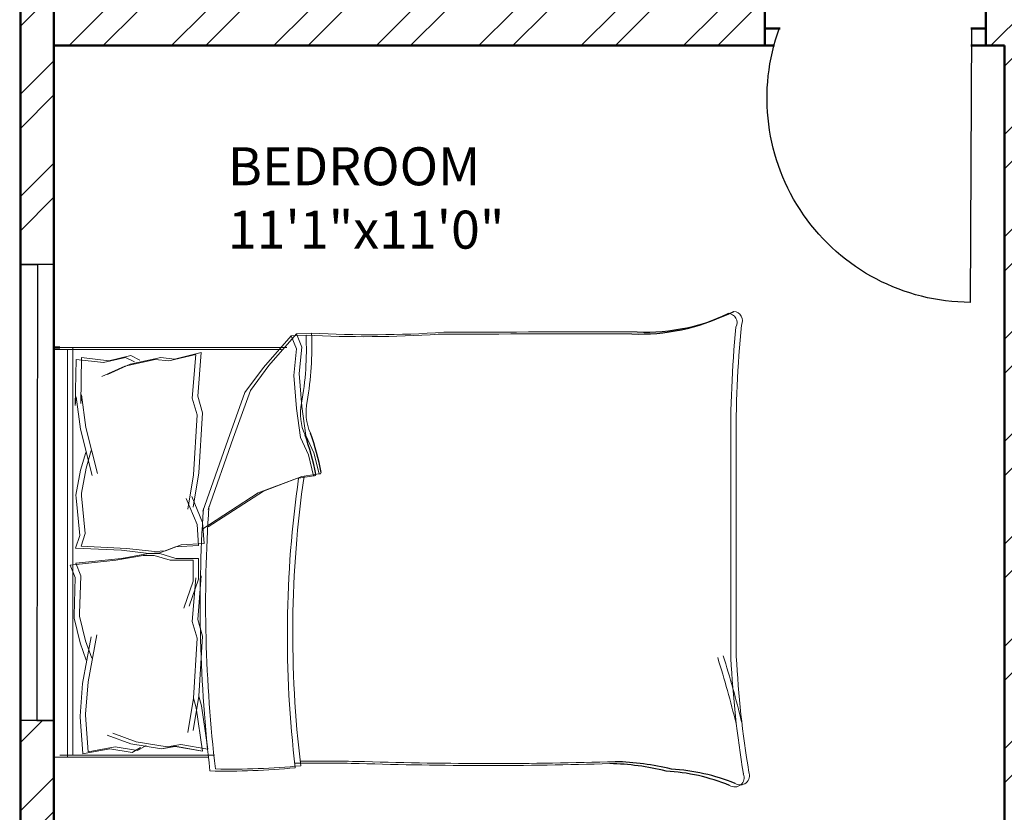
# Model space of a CAD drawing. Units: inches. Extents: x 1901 to 2863, y 888 to 2433.
# Tile 3 of 91: x 2025 to 2154, y 1338 to 1442. Entities that reach past the tile are written whole.
import ezdxf

# ---------------------------------------------------------------- set-up
doc = ezdxf.new("R2010")
doc.units = ezdxf.units.IN
for name, color, linetype, lineweight in [('A-AREA-IDEN', 7, 'Continuous', 18), ('A-DOOR', 4, 'Continuous', 25), ('A-FURN', 8, 'Continuous', 18), ('A-GLAZ', 3, 'Continuous', 25), ('A-WALL', 7, 'Continuous', 50), ('A-WALL-PATT', 8, 'Continuous', 13)]:
    doc.layers.add(name, color=color, linetype=linetype, lineweight=lineweight)
doc.styles.get("Standard").update_dxf_attribs({"font": 'arial.ttf'})

# ---------------------------------------------------------------- blocks, each defined once
blk = doc.blocks.new('WIN-60')
for p, q in [((0, 4.5), (0, 0)), ((60, 2.25), (60, 4.5)), ((60, 4.5), (60, 0)), ((0, 0), (0, 2.25)), ((0, 2.25), (60, 2.25))]:
    blk.add_line(p, q)
blk = doc.blocks.new('DOOR-27')
blk.add_line((26.81, -0.02), (26.81, 35.98))
blk.add_arc((26.81, 9.12), 26.86, 90, 199.8893)

msp = doc.modelspace()

# ---------------------------------------------------------------- hatches: boundary and pattern name
at = {"layer": 'A-WALL-PATT'}
h = msp.add_hatch(dxfattribs=at)
h.set_pattern_fill('ANSI32', color=256)
h.paths.add_polyline_path([(2192.5, 2274.13), (2141.26, 2274.13), (2141.26, 2269.63), (2192.5, 2269.63)])
h.paths.add_polyline_path([(2259.93, 2274.13), (2216.5, 2274.13), (2216.5, 2269.63), (2255.43, 2269.63), (2255.43, 2214.63), (2250.81, 2214.63), (2250.81, 2210.13), (2259.93, 2210.13), (2259.93, 2215.13), (2271.76, 2215.13), (2271.76, 2217.38), (2271.76, 2219.63), (2259.93, 2219.63)])
h.paths.add_polyline_path([(2171.43, 2269.63), (2166.93, 2269.63), (2166.93, 2219.63), (2121.24, 2219.63), (2121.24, 2215.13), (2166.93, 2215.13), (2166.93, 2083.13), (2161.81, 2083.13), (2161.81, 2078.63), (2171.43, 2078.63), (2177, 2078.63), (2177, 2080.88), (2177, 2083.13), (2171.43, 2083.13), (2171.43, 2210.13), (2230.91, 2210.13), (2230.91, 2212.38), (2230.91, 2214.63), (2171.43, 2214.63)])
h.paths.add_polyline_path([(2117.26, 2274.13), (2089.43, 2274.13), (2089.43, 2219.63), (2081.14, 2219.63), (2081.14, 2215.13), (2089.43, 2215.13), (2098, 2215.13), (2098, 2217.38), (2098, 2219.63), (2093.93, 2219.63), (2093.93, 2269.63), (2117.26, 2269.63), (2117.26, 2271.88)])
h.paths.add_polyline_path([(2343.43, 2219.63), (2329.29, 2219.63), (2329.29, 2215.13), (2338.93, 2215.13), (2338.93, 2184.74), (2343.43, 2184.74)])
h.paths.add_polyline_path([(2338.93, 2083.13), (2329.29, 2083.13), (2208.97, 2083.13), (2208.97, 2078.63), (2338.93, 2078.63)])
h.paths.add_polyline_path([(2343.43, 2136.74), (2338.93, 2136.74), (2338.93, 1872.63), (2343.43, 1872.63)])
h.paths.add_polyline_path([(2343.43, 1863.63), (2397.68, 1863.63), (2397.68, 1821.63), (2384.14, 1821.63), (2384.14, 1812.63), (2418.33, 1812.63), (2418.33, 1817.13), (2418.33, 1821.63), (2406.68, 1821.63), (2406.68, 1863.63), (2459.5, 1863.63), (2459.5, 1821.63), (2447.14, 1821.63), (2447.14, 1812.63), (2459.5, 1812.63), (2468.5, 1812.63), (2468.5, 1872.63), (2394.43, 1872.63), (2334.43, 1872.63), (2334.43, 1812.63), (2343.43, 1812.63), (2353.25, 1812.63), (2353.25, 1821.63), (2343.43, 1821.63)])
h.paths.add_polyline_path([(2510.01, 1872.63), (2468.5, 1872.63), (2468.5, 1868.13), (2510.01, 1868.13)])
h.paths.add_polyline_path([(2514.01, 1817.13), (2468.5, 1817.13), (2468.5, 1812.63), (2482.11, 1812.63), (2482.11, 1800.61), (2486.61, 1800.61), (2486.61, 1812.63), (2514.01, 1812.63)])
h.paths.add_polyline_path([(2299.25, 1814.88), (2299.25, 1817.13), (2295.93, 1817.13), (2295.93, 1854.17), (2293.68, 1854.17), (2291.43, 1854.17), (2291.43, 1817.13), (2266.11, 1817.13), (2266.11, 1812.63), (2299.25, 1812.63)])
h.paths.add_polyline_path([(2218.11, 1817.13), (2206.46, 1817.13), (2171.43, 1817.13), (2171.43, 1949.13), (2190.1, 1949.13), (2190.1, 1953.63), (2163.47, 1953.63), (2163.47, 1949.13), (2166.93, 1949.13), (2166.93, 1817.13), (2114.3, 1817.13), (2114.3, 1812.63), (2218.11, 1812.63)])
h.paths.add_polyline_path([(2029.43, 1970.92), (2024.93, 1970.92), (2024.93, 1912.72), (2029.43, 1912.72)])
h.paths.add_polyline_path([(2132.3, 1953.63), (2113.93, 1953.63), (2113.93, 1975.89), (2111.68, 1975.89), (2109.43, 1975.89), (2109.43, 1953.63), (2029.43, 1953.63), (2029.43, 1949.13), (2132.3, 1949.13)])
h.paths.add_polyline_path([(2029.43, 1853.61), (2029.31, 1853.61), (2029.31, 1853.61), (2029.43, 1853.61), (2029.43, 1864.72), (2024.93, 1864.72), (2024.93, 1812.63), (2066.3, 1812.63), (2066.3, 1814.88), (2066.3, 1817.13), (2029.43, 1817.13)])
h.paths.add_polyline_path([(2122.93, 2010.09), (2120.68, 2010.09), (2118.43, 2010.09), (2118.43, 2006.13), (2029.43, 2006.13), (2029.43, 2001.63), (2109.43, 2001.63), (2109.43, 1998.04), (2113.93, 1998.04), (2113.93, 2001.63), (2122.93, 2001.63)])
h.paths.add_polyline_path([(2029.43, 2031.38), (2024.93, 2031.38), (2024.93, 1994.92), (2027.18, 1994.92), (2029.43, 1994.92)])
h.paths.add_polyline_path([(2029.43, 2136.74), (2024.93, 2136.74), (2024.93, 2067.38), (2027.18, 2067.38), (2029.43, 2067.38)])
h.paths.add_polyline_path([(2125.62, 2083.13), (2029.43, 2083.13), (2029.43, 2078.63), (2118.43, 2078.63), (2118.43, 2030.71), (2122.93, 2030.71), (2122.93, 2078.63), (2125.62, 2078.63)])
h.paths.add_polyline_path([(2029.43, 2215.13), (2040.47, 2215.13), (2040.47, 2217.38), (2040.47, 2219.63), (2024.93, 2219.63), (2024.93, 2184.74), (2029.43, 2184.74), (2029.43, 2187.78)])
h.paths.add_polyline_path([(2686.43, 2274.13), (2659.28, 2274.13), (2659.28, 2269.63), (2681.93, 2269.63), (2681.93, 2219.63), (2676.82, 2219.63), (2676.82, 2215.13), (2681.93, 2215.13), (2697.01, 2215.13), (2697.01, 2217.38), (2697.01, 2219.63), (2686.43, 2219.63)])
h.paths.add_polyline_path([(2609.93, 2269.63), (2635.28, 2269.63), (2635.28, 2274.13), (2571.43, 2274.13), (2571.43, 2269.63), (2605.43, 2269.63), (2605.43, 2214.63), (2549.1, 2214.63), (2549.1, 2210.13), (2605.43, 2210.13), (2605.43, 2083.13), (2601.01, 2083.13), (2601.01, 2080.88), (2601.01, 2078.63), (2609.93, 2078.63), (2616.16, 2078.63), (2616.16, 2080.88), (2616.16, 2083.13), (2609.93, 2083.13), (2609.93, 2215.13), (2651.46, 2215.13), (2651.46, 2217.38), (2651.46, 2219.63), (2609.93, 2219.63)])
h.paths.add_polyline_path([(2521.43, 2269.63), (2547.43, 2269.63), (2547.43, 2271.88), (2547.43, 2274.13), (2516.93, 2274.13), (2516.93, 2219.63), (2506.41, 2219.63), (2506.41, 2215.13), (2516.93, 2215.13), (2516.93, 2210.13), (2525.4, 2210.13), (2525.4, 2212.38), (2525.4, 2214.63), (2521.43, 2214.63)])
h.paths.add_polyline_path([(2456.01, 2219.63), (2439.43, 2219.63), (2439.43, 2187.89), (2443.93, 2187.89), (2443.93, 2215.13), (2456.01, 2215.13)])
h.paths.add_polyline_path([(2752.93, 2219.63), (2739.48, 2219.63), (2739.48, 2215.13), (2748.43, 2215.13), (2748.43, 2187.89), (2752.93, 2187.89)])
h.paths.add_polyline_path([(2752.93, 2139.89), (2748.43, 2139.89), (2748.43, 2083.13), (2648.42, 2083.13), (2648.42, 2078.63), (2654.93, 2078.63), (2654.93, 2039.44), (2659.43, 2039.44), (2659.43, 2078.63), (2748.43, 2078.63), (2748.43, 2063.43), (2752.93, 2063.43)])
h.paths.add_polyline_path([(2752.93, 2010.63), (2659.43, 2010.63), (2659.43, 2015.65), (2654.93, 2015.65), (2654.93, 2010.63), (2605.43, 2010.63), (2605.43, 1920.97), (2609.93, 1920.97), (2609.93, 2006.13), (2748.43, 2006.13), (2748.43, 1982.47), (2752.93, 1982.47)])
h.paths.add_polyline_path([(2752.93, 2027.43), (2748.43, 2027.43), (2748.43, 2010.63), (2752.93, 2010.63)])
h.paths.add_polyline_path([(2748.43, 1886.13), (2609.93, 1886.13), (2609.93, 1889.72), (2605.43, 1889.72), (2605.43, 1861.26), (2609.93, 1861.26), (2609.93, 1881.63), (2748.43, 1881.63)])
h.paths.add_polyline_path([(2456.86, 2228.83), (2498.4, 2228.83), (2498.4, 2247.49), (2456.86, 2247.49)], flags=9)
h.paths.add_polyline_path([(2038.6, 2237.42), (2080.17, 2237.42), (2080.17, 2256.08), (2038.6, 2256.08)], flags=9)
h.paths.add_polyline_path([(2292.01, 1062.39), (2539.93, 1062.39), (2539.93, 1099.49), (2292.01, 1099.49)], flags=9)
h.paths.add_polyline_path([(2424.91, 1832.25), (2448.51, 1832.25), (2448.51, 1846.68), (2424.91, 1846.68)], flags=25)
h.paths.add_polyline_path([(2359.08, 1832.25), (2382.68, 1832.25), (2382.68, 1846.68), (2359.08, 1846.68)], flags=25)
h.paths.add_polyline_path([(2352.9, 1684.8), (2367.54, 1684.8), (2367.54, 1697.17), (2352.9, 1697.17)], flags=9)
h.paths.add_polyline_path([(2079.29, 1755.83), (2169.02, 1755.83), (2169.02, 1774.37), (2079.29, 1774.37)], flags=9)
h.paths.add_polyline_path([(2404.09, 1373.86), (2404.09, 1463.59), (2385.54, 1463.59), (2385.54, 1373.86)], flags=9)
h.paths.add_polyline_path([(2268.09, 2236.37), (2309.64, 2236.37), (2309.64, 2255.03), (2268.09, 2255.03)], flags=9)
h.paths.add_polyline_path([(2575.96, 1700.95), (2665.7, 1700.95), (2665.7, 1719.5), (2575.96, 1719.5)], flags=9)
h.paths.add_polyline_path([(2302.96, 1878.47), (2329.52, 1878.47), (2329.52, 1888.78), (2302.96, 1888.78)], flags=9)
h.paths.add_polyline_path([(2097.42, 2240.58), (2126.57, 2240.58), (2126.57, 2259.23), (2097.42, 2259.23)], flags=9)
h.paths.add_polyline_path([(2208.72, 2246.12), (2237.88, 2246.12), (2237.88, 2264.78), (2208.72, 2264.78)], flags=9)
h.paths.add_polyline_path([(2038.15, 1925.96), (2076.99, 1925.96), (2076.99, 1944.62), (2038.15, 1944.62)], flags=9)
h.paths.add_polyline_path([(2239.14, 1926.67), (2288.46, 1926.67), (2288.46, 1945.33), (2239.14, 1945.33)], flags=9)
h.paths.add_polyline_path([(2175.43, 2007.33), (2212.36, 2007.33), (2212.36, 2025.99), (2175.43, 2025.99)], flags=9)
h.paths.add_polyline_path([(2225.03, 2091.79), (2263.87, 2091.79), (2263.87, 2110.45), (2225.03, 2110.45)], flags=9)
h.paths.add_polyline_path([(2035.4, 2098.48), (2074.24, 2098.48), (2074.24, 2117.14), (2035.4, 2117.14)], flags=9)
h.paths.add_polyline_path([(2050.1, 2029.21), (2083.26, 2029.21), (2083.26, 2047.87), (2050.1, 2047.87)], flags=9)
h.paths.add_polyline_path([(2069.68, 1956.72), (2098.83, 1956.72), (2098.83, 1975.38), (2069.68, 1975.38)], flags=25)
h.paths.add_polyline_path([(2328.62, 1753.34), (2361.66, 1753.34), (2361.66, 1771.99), (2328.62, 1771.99)], flags=9)
h.paths.add_polyline_path([(2395.16, 2060.89), (2395.16, 2140.65), (2378.68, 2140.65), (2378.68, 2060.89)], flags=9)
h.paths.add_polyline_path([(2463.73, 2059.02), (2492.89, 2059.02), (2492.89, 2077.68), (2463.73, 2077.68)], flags=9)
h.paths.add_polyline_path([(2458.03, 2181.54), (2496.87, 2181.54), (2496.87, 2200.19), (2458.03, 2200.19)], flags=9)
h.paths.add_polyline_path([(2527.58, 2243.07), (2556.73, 2243.07), (2556.73, 2261.73), (2527.58, 2261.73)], flags=9)
h.paths.add_polyline_path([(2694.46, 2232.77), (2736.03, 2232.77), (2736.03, 2251.42), (2694.46, 2251.42)], flags=9)
h.paths.add_polyline_path([(2637.82, 2249.22), (2666.98, 2249.22), (2666.98, 2267.88), (2637.82, 2267.88)], flags=9)
h.paths.add_polyline_path([(2623.69, 2183.54), (2662.53, 2183.54), (2662.53, 2202.2), (2623.69, 2202.2)], flags=9)
h.paths.add_polyline_path([(2691.97, 2021.5), (2725.12, 2021.5), (2725.12, 2040.16), (2691.97, 2040.16)], flags=9)
h.paths.add_polyline_path([(2621.04, 1975.91), (2662.34, 1975.91), (2662.34, 1994.57), (2621.04, 1994.57)], flags=25)
h.paths.add_polyline_path([(2479.03, 1927.62), (2519.84, 1927.62), (2519.84, 1946.28), (2479.03, 1946.28)], flags=9)
h.paths.add_polyline_path([(2670.94, 1849.08), (2716.01, 1849.08), (2716.01, 1867.73), (2670.94, 1867.73)], flags=9)
h.paths.add_polyline_path([(2523.61, 1782.96), (2550.17, 1782.96), (2550.17, 1793.26), (2523.61, 1793.26)], flags=9)
h.paths.add_polyline_path([(2450.84, 1207.33), (2492.39, 1207.33), (2492.39, 1225.99), (2450.84, 1225.99)], flags=9)
h.paths.add_polyline_path([(2527.75, 1203.84), (2556.91, 1203.84), (2556.91, 1222.5), (2527.75, 1222.5)], flags=9)
h.paths.add_polyline_path([(2639.11, 1207.2), (2668.27, 1207.2), (2668.27, 1225.86), (2639.11, 1225.86)], flags=9)
h.paths.add_polyline_path([(2692.59, 1218.97), (2734.17, 1218.97), (2734.17, 1237.62), (2692.59, 1237.62)], flags=9)
h.paths.add_polyline_path([(2669.27, 1366.33), (2708.11, 1366.33), (2708.11, 1384.99), (2669.27, 1384.99)], flags=9)
h.paths.add_polyline_path([(2463.31, 1358.03), (2502.15, 1358.03), (2502.15, 1376.69), (2463.31, 1376.69)], flags=9)
h.paths.add_polyline_path([(2494.72, 1449.96), (2531.65, 1449.96), (2531.65, 1468.62), (2494.72, 1468.62)], flags=9)
h.paths.add_polyline_path([(2675.57, 1422.16), (2708.72, 1422.16), (2708.72, 1440.81), (2675.57, 1440.81)], flags=9)
h.paths.add_polyline_path([(2685.63, 1493.89), (2714.79, 1493.89), (2714.79, 1512.55), (2685.63, 1512.55)], flags=9)
h.paths.add_polyline_path([(2686.8, 1529.91), (2725.65, 1529.91), (2725.65, 1548.57), (2686.8, 1548.57)], flags=9)
h.paths.add_polyline_path([(2503.65, 1537.99), (2552.97, 1537.99), (2552.97, 1556.65), (2503.65, 1556.65)], flags=9)
h.paths.add_polyline_path([(2291.71, 1643.5), (2318.28, 1643.5), (2318.28, 1653.81), (2291.71, 1653.81)], flags=9)
h.paths.add_polyline_path([(2450.63, 1610.52), (2477.19, 1610.52), (2477.19, 1620.82), (2450.63, 1620.82)], flags=9)
h.paths.add_polyline_path([(2359.99, 1551.81), (2422.25, 1551.81), (2422.25, 1562.12), (2359.99, 1562.12)], flags=9)
h.paths.add_polyline_path([(2280.11, 1249.01), (2321.65, 1249.01), (2321.65, 1267.66), (2280.11, 1267.66)], flags=9)
h.paths.add_polyline_path([(2164.06, 1274.23), (2193.22, 1274.23), (2193.22, 1292.89), (2164.06, 1292.89)], flags=9)
h.paths.add_polyline_path([(2118.21, 1277.69), (2151.25, 1277.69), (2151.25, 1296.35), (2118.21, 1296.35)], flags=9)
h.paths.add_polyline_path([(2031.95, 1268.53), (2073.52, 1268.53), (2073.52, 1287.19), (2031.95, 1287.19)], flags=9)
h.paths.add_polyline_path([(2050.2, 1409.08), (2089.04, 1409.08), (2089.04, 1427.74), (2050.2, 1427.74)], flags=9)
h.paths.add_polyline_path([(2243.74, 1421.03), (2282.58, 1421.03), (2282.58, 1439.69), (2243.74, 1439.69)], flags=9)
h.paths.add_polyline_path([(2190.75, 1509.77), (2231.56, 1509.77), (2231.56, 1528.43), (2190.75, 1528.43)], flags=9)
h.paths.add_polyline_path([(2058.39, 1475.42), (2091.55, 1475.42), (2091.55, 1494.07), (2058.39, 1494.07)], flags=9)
h.paths.add_polyline_path([(2062.45, 1553.09), (2091.6, 1553.09), (2091.6, 1571.75), (2062.45, 1571.75)], flags=9)
h.paths.add_polyline_path([(2219.52, 1590.37), (2266.15, 1590.37), (2266.15, 1609.02), (2219.52, 1609.02)], flags=9)
h.paths.add_polyline_path([(2041.07, 1584.19), (2079.91, 1584.19), (2079.91, 1602.85), (2041.07, 1602.85)], flags=9)
h = msp.add_hatch(dxfattribs=at)
h.set_pattern_fill('ANSI32', color=256)
h.paths.add_polyline_path([(2443.93, 2139.89), (2439.43, 2139.89), (2439.43, 2069.35), (2441.68, 2069.35), (2443.93, 2069.35), (2443.93, 2078.63), (2521.93, 2078.63), (2521.93, 2075.07), (2524.18, 2075.07), (2526.43, 2075.07), (2526.43, 2078.63), (2571.75, 2078.63), (2571.75, 2080.88), (2571.75, 2083.13), (2443.93, 2083.13)])
h.paths.add_polyline_path([(2526.43, 2054.63), (2524.18, 2054.63), (2521.93, 2054.63), (2521.93, 2030.63), (2443.93, 2030.63), (2443.93, 2045.35), (2439.43, 2045.35), (2439.43, 1983.87), (2443.93, 1983.87), (2443.93, 2026.13), (2521.93, 2026.13), (2526.43, 2026.13)])
h.paths.add_polyline_path([(2443.93, 1923.87), (2439.43, 1923.87), (2439.43, 1872.63), (2443.93, 1872.63)])
h.paths.add_polyline_path([(2636.23, 1766.13), (2609.93, 1766.13), (2609.93, 1779.79), (2605.43, 1779.79), (2605.43, 1766.13), (2486.61, 1766.13), (2486.61, 1770.67), (2482.11, 1770.67), (2482.11, 1766.13), (2482.11, 1761.63), (2636.23, 1761.63), (2636.23, 1763.88)])
h.paths.add_polyline_path([(2519.54, 1663.38), (2519.54, 1665.63), (2494.93, 1665.63), (2481.83, 1665.63), (2481.83, 1663.38), (2481.83, 1661.13), (2490.43, 1661.13), (2490.43, 1640.16), (2494.93, 1640.16), (2494.93, 1661.13), (2519.54, 1661.13)])
h.paths.add_polyline_path([(2443.93, 1712.13), (2443.93, 1716.63), (2414.46, 1716.63), (2414.46, 1712.13), (2439.43, 1712.13), (2439.43, 1545.51), (2443.93, 1545.51), (2443.93, 1661.13), (2448.47, 1661.13), (2448.47, 1665.63), (2443.93, 1665.63)])
h.paths.add_polyline_path([(2343.43, 1712.13), (2365.52, 1712.13), (2365.52, 1714.38), (2365.52, 1716.63), (2333.87, 1716.63), (2333.87, 1714.38), (2333.87, 1712.13), (2338.93, 1712.13), (2338.93, 1575.63), (2338.93, 1545.51), (2343.43, 1545.51), (2343.43, 1547.51), (2343.43, 1580.13)])
h.paths.add_polyline_path([(2752.93, 1665.63), (2579.54, 1665.63), (2579.54, 1661.13), (2615.93, 1661.13), (2615.93, 1529.13), (2598.93, 1529.13), (2598.93, 1524.63), (2623.13, 1524.63), (2623.13, 1526.88), (2623.13, 1529.13), (2620.43, 1529.13), (2620.43, 1661.13), (2748.43, 1661.13), (2748.43, 1633.5), (2752.93, 1633.5)])
h.paths.add_polyline_path([(2752.93, 1419.93), (2748.43, 1419.93), (2748.43, 1400.13), (2659.43, 1400.13), (2659.43, 1444.33), (2657.18, 1444.33), (2654.93, 1444.33), (2654.93, 1400.13), (2643.65, 1400.13), (2643.65, 1395.63), (2748.43, 1395.63), (2748.43, 1364.04), (2752.93, 1364.04)])
h.paths.add_polyline_path([(2752.93, 1492.88), (2748.43, 1492.88), (2748.43, 1476.63), (2667.43, 1476.63), (2667.43, 1479.71), (2665.18, 1479.71), (2662.93, 1479.71), (2662.93, 1476.63), (2654.93, 1476.63), (2654.93, 1469.54), (2659.43, 1469.54), (2659.43, 1472.13), (2748.43, 1472.13), (2748.43, 1455.93), (2752.93, 1455.93)])
h.paths.add_polyline_path([(2752.93, 1304.04), (2748.43, 1304.04), (2748.43, 1263.63), (2738.66, 1263.63), (2738.66, 1259.13), (2752.93, 1259.13)])
h.paths.add_polyline_path([(2685.93, 1259.13), (2695.49, 1259.13), (2695.49, 1261.38), (2695.49, 1263.63), (2677.84, 1263.63), (2677.84, 1261.38), (2677.84, 1259.13), (2681.43, 1259.13), (2681.43, 1203.63), (2653.28, 1203.63), (2653.28, 1199.13), (2685.93, 1199.13), (2685.93, 1203.63)])
h.paths.add_polyline_path([(2609.43, 1395.63), (2611.85, 1395.63), (2611.85, 1400.13), (2598.89, 1400.13), (2598.89, 1397.88), (2598.89, 1395.63), (2604.93, 1395.63), (2604.93, 1268.13), (2554.73, 1268.13), (2554.73, 1265.88), (2554.73, 1263.63), (2604.93, 1263.63), (2604.93, 1203.63), (2571.31, 1203.63), (2571.31, 1199.13), (2604.93, 1199.13), (2629.28, 1199.13), (2629.28, 1201.38), (2629.28, 1203.63), (2609.43, 1203.63), (2609.43, 1258.63), (2609.43, 1259.13), (2654.8, 1259.13), (2654.8, 1263.63), (2609.43, 1263.63)])
h.paths.add_polyline_path([(2443.93, 1304.04), (2439.43, 1304.04), (2439.43, 1259.13), (2443.93, 1259.13), (2456.16, 1259.13), (2456.16, 1261.38), (2456.16, 1263.63), (2443.93, 1263.63)])
h.paths.add_polyline_path([(2525.43, 1263.63), (2531.78, 1263.63), (2531.78, 1268.13), (2520.93, 1268.13), (2520.93, 1263.63), (2511.41, 1263.63), (2511.41, 1259.13), (2520.93, 1259.13), (2520.93, 1199.13), (2547.31, 1199.13), (2547.31, 1201.38), (2547.31, 1203.63), (2525.43, 1203.63)])
h.paths.add_polyline_path([(2443.93, 1434.84), (2439.43, 1434.84), (2439.43, 1364.04), (2441.68, 1364.04), (2443.93, 1364.04)])
h.paths.add_polyline_path([(2567.13, 1400.13), (2443.93, 1400.13), (2443.93, 1395.63), (2567.13, 1395.63)])
h.paths.add_polyline_path([(2443.93, 1545.51), (2439.43, 1545.51), (2439.43, 1494.84), (2443.93, 1494.84)])
h.paths.add_polyline_path([(2494.93, 1553.35), (2492.68, 1553.35), (2490.43, 1553.35), (2490.43, 1524.63), (2494.93, 1524.63), (2525.94, 1524.63), (2525.94, 1526.88), (2525.94, 1529.13), (2494.93, 1529.13)])
h.paths.add_polyline_path([(2752.93, 1573.5), (2748.43, 1573.5), (2748.43, 1529.13), (2657.76, 1529.13), (2657.76, 1524.63), (2662.93, 1524.63), (2662.93, 1498.63), (2667.43, 1498.63), (2667.43, 1524.63), (2748.43, 1524.63), (2748.43, 1516.88), (2752.93, 1516.88)])
h.paths.add_polyline_path([(2038.6, 2237.42), (2080.17, 2237.42), (2080.17, 2256.08), (2038.6, 2256.08)], flags=9)
h.paths.add_polyline_path([(2292.01, 1062.39), (2539.93, 1062.39), (2539.93, 1099.49), (2292.01, 1099.49)], flags=9)
h.paths.add_polyline_path([(2424.91, 1832.25), (2448.51, 1832.25), (2448.51, 1846.68), (2424.91, 1846.68)], flags=9)
h.paths.add_polyline_path([(2359.08, 1832.25), (2382.68, 1832.25), (2382.68, 1846.68), (2359.08, 1846.68)], flags=9)
h.paths.add_polyline_path([(2352.9, 1684.8), (2367.54, 1684.8), (2367.54, 1697.17), (2352.9, 1697.17)], flags=9)
h.paths.add_polyline_path([(2079.29, 1755.83), (2169.02, 1755.83), (2169.02, 1774.37), (2079.29, 1774.37)], flags=9)
h.paths.add_polyline_path([(2404.09, 1373.86), (2404.09, 1463.59), (2385.54, 1463.59), (2385.54, 1373.86)], flags=9)
h.paths.add_polyline_path([(2268.09, 2236.37), (2309.64, 2236.37), (2309.64, 2255.03), (2268.09, 2255.03)], flags=9)
h.paths.add_polyline_path([(2575.96, 1700.95), (2665.7, 1700.95), (2665.7, 1719.5), (2575.96, 1719.5)], flags=9)
h.paths.add_polyline_path([(2302.96, 1878.47), (2329.52, 1878.47), (2329.52, 1888.78), (2302.96, 1888.78)], flags=9)
h.paths.add_polyline_path([(2097.42, 2240.58), (2126.57, 2240.58), (2126.57, 2259.23), (2097.42, 2259.23)], flags=9)
h.paths.add_polyline_path([(2208.72, 2246.12), (2237.88, 2246.12), (2237.88, 2264.78), (2208.72, 2264.78)], flags=9)
h.paths.add_polyline_path([(2038.15, 1925.96), (2076.99, 1925.96), (2076.99, 1944.62), (2038.15, 1944.62)], flags=9)
h.paths.add_polyline_path([(2239.14, 1926.67), (2288.46, 1926.67), (2288.46, 1945.33), (2239.14, 1945.33)], flags=9)
h.paths.add_polyline_path([(2175.43, 2007.33), (2212.36, 2007.33), (2212.36, 2025.99), (2175.43, 2025.99)], flags=9)
h.paths.add_polyline_path([(2225.03, 2091.79), (2263.87, 2091.79), (2263.87, 2110.45), (2225.03, 2110.45)], flags=9)
h.paths.add_polyline_path([(2035.4, 2098.48), (2074.24, 2098.48), (2074.24, 2117.14), (2035.4, 2117.14)], flags=9)
h.paths.add_polyline_path([(2050.1, 2029.21), (2083.26, 2029.21), (2083.26, 2047.87), (2050.1, 2047.87)], flags=9)
h.paths.add_polyline_path([(2069.68, 1956.72), (2098.83, 1956.72), (2098.83, 1975.38), (2069.68, 1975.38)], flags=9)
h.paths.add_polyline_path([(2328.62, 1753.34), (2361.66, 1753.34), (2361.66, 1771.99), (2328.62, 1771.99)], flags=9)
h.paths.add_polyline_path([(2395.16, 2060.89), (2395.16, 2140.65), (2378.68, 2140.65), (2378.68, 2060.89)], flags=9)
h.paths.add_polyline_path([(2463.73, 2059.02), (2492.89, 2059.02), (2492.89, 2077.68), (2463.73, 2077.68)], flags=9)
h.paths.add_polyline_path([(2458.03, 2181.54), (2496.87, 2181.54), (2496.87, 2200.19), (2458.03, 2200.19)], flags=9)
h.paths.add_polyline_path([(2456.86, 2228.83), (2498.4, 2228.83), (2498.4, 2247.49), (2456.86, 2247.49)], flags=9)
h.paths.add_polyline_path([(2527.58, 2243.07), (2556.73, 2243.07), (2556.73, 2261.73), (2527.58, 2261.73)], flags=9)
h.paths.add_polyline_path([(2694.46, 2232.77), (2736.03, 2232.77), (2736.03, 2251.42), (2694.46, 2251.42)], flags=9)
h.paths.add_polyline_path([(2637.82, 2249.22), (2666.98, 2249.22), (2666.98, 2267.88), (2637.82, 2267.88)], flags=9)
h.paths.add_polyline_path([(2623.69, 2183.54), (2662.53, 2183.54), (2662.53, 2202.2), (2623.69, 2202.2)], flags=9)
h.paths.add_polyline_path([(2691.97, 2021.5), (2725.12, 2021.5), (2725.12, 2040.16), (2691.97, 2040.16)], flags=9)
h.paths.add_polyline_path([(2621.04, 1975.91), (2662.34, 1975.91), (2662.34, 1994.57), (2621.04, 1994.57)], flags=9)
h.paths.add_polyline_path([(2479.03, 1927.62), (2519.84, 1927.62), (2519.84, 1946.28), (2479.03, 1946.28)], flags=9)
h.paths.add_polyline_path([(2670.94, 1849.08), (2716.01, 1849.08), (2716.01, 1867.73), (2670.94, 1867.73)], flags=9)
h.paths.add_polyline_path([(2523.61, 1782.96), (2550.17, 1782.96), (2550.17, 1793.26), (2523.61, 1793.26)], flags=9)
h.paths.add_polyline_path([(2450.84, 1207.33), (2492.39, 1207.33), (2492.39, 1225.99), (2450.84, 1225.99)], flags=9)
h.paths.add_polyline_path([(2527.75, 1203.84), (2556.91, 1203.84), (2556.91, 1222.5), (2527.75, 1222.5)], flags=9)
h.paths.add_polyline_path([(2639.11, 1207.2), (2668.27, 1207.2), (2668.27, 1225.86), (2639.11, 1225.86)], flags=9)
h.paths.add_polyline_path([(2692.59, 1218.97), (2734.17, 1218.97), (2734.17, 1237.62), (2692.59, 1237.62)], flags=9)
h.paths.add_polyline_path([(2669.27, 1366.33), (2708.11, 1366.33), (2708.11, 1384.99), (2669.27, 1384.99)], flags=25)
h.paths.add_polyline_path([(2463.31, 1358.03), (2502.15, 1358.03), (2502.15, 1376.69), (2463.31, 1376.69)], flags=9)
h.paths.add_polyline_path([(2494.72, 1449.96), (2531.65, 1449.96), (2531.65, 1468.62), (2494.72, 1468.62)], flags=9)
h.paths.add_polyline_path([(2675.57, 1422.16), (2708.72, 1422.16), (2708.72, 1440.81), (2675.57, 1440.81)], flags=25)
h.paths.add_polyline_path([(2685.63, 1493.89), (2714.79, 1493.89), (2714.79, 1512.55), (2685.63, 1512.55)], flags=9)
h.paths.add_polyline_path([(2686.8, 1529.91), (2725.65, 1529.91), (2725.65, 1548.57), (2686.8, 1548.57)], flags=25)
h.paths.add_polyline_path([(2503.65, 1537.99), (2552.97, 1537.99), (2552.97, 1556.65), (2503.65, 1556.65)], flags=9)
h.paths.add_polyline_path([(2291.71, 1643.5), (2318.28, 1643.5), (2318.28, 1653.81), (2291.71, 1653.81)], flags=9)
h.paths.add_polyline_path([(2450.63, 1610.52), (2477.19, 1610.52), (2477.19, 1620.82), (2450.63, 1620.82)], flags=9)
h.paths.add_polyline_path([(2359.99, 1551.81), (2422.25, 1551.81), (2422.25, 1562.12), (2359.99, 1562.12)], flags=9)
h.paths.add_polyline_path([(2280.11, 1249.01), (2321.65, 1249.01), (2321.65, 1267.66), (2280.11, 1267.66)], flags=9)
h.paths.add_polyline_path([(2164.06, 1274.23), (2193.22, 1274.23), (2193.22, 1292.89), (2164.06, 1292.89)], flags=9)
h.paths.add_polyline_path([(2118.21, 1277.69), (2151.25, 1277.69), (2151.25, 1296.35), (2118.21, 1296.35)], flags=9)
h.paths.add_polyline_path([(2031.95, 1268.53), (2073.52, 1268.53), (2073.52, 1287.19), (2031.95, 1287.19)], flags=9)
h.paths.add_polyline_path([(2050.2, 1409.08), (2089.04, 1409.08), (2089.04, 1427.74), (2050.2, 1427.74)], flags=9)
h.paths.add_polyline_path([(2243.74, 1421.03), (2282.58, 1421.03), (2282.58, 1439.69), (2243.74, 1439.69)], flags=9)
h.paths.add_polyline_path([(2190.75, 1509.77), (2231.56, 1509.77), (2231.56, 1528.43), (2190.75, 1528.43)], flags=9)
h.paths.add_polyline_path([(2058.39, 1475.42), (2091.55, 1475.42), (2091.55, 1494.07), (2058.39, 1494.07)], flags=9)
h.paths.add_polyline_path([(2062.45, 1553.09), (2091.6, 1553.09), (2091.6, 1571.75), (2062.45, 1571.75)], flags=9)
h.paths.add_polyline_path([(2219.52, 1590.37), (2266.15, 1590.37), (2266.15, 1609.02), (2219.52, 1609.02)], flags=9)
h.paths.add_polyline_path([(2041.07, 1584.19), (2079.91, 1584.19), (2079.91, 1602.85), (2041.07, 1602.85)], flags=9)
h = msp.add_hatch(dxfattribs=at)
h.set_pattern_fill('ANSI32', color=256)
h.paths.add_polyline_path([(2182.93, 1716.63), (2024.93, 1716.63), (2024.93, 1681.7), (2029.33, 1681.7), (2029.33, 1712.13), (2154.33, 1712.13), (2154.33, 1580.13), (2148.52, 1580.13), (2148.52, 1577.88), (2148.52, 1575.63), (2194.93, 1575.63), (2194.93, 1580.13), (2158.83, 1580.13), (2158.83, 1712.13), (2182.93, 1712.13)])
h.paths.add_polyline_path([(2301.07, 1716.63), (2242.93, 1716.63), (2242.93, 1712.13), (2283.83, 1712.13), (2283.83, 1685.54), (2288.33, 1685.54), (2288.33, 1712.13), (2301.07, 1712.13)])
h.paths.add_polyline_path([(2288.33, 1600.41), (2286.08, 1600.41), (2283.83, 1600.41), (2283.83, 1580.13), (2270.6, 1580.13), (2270.6, 1575.63), (2288.33, 1575.63)])
h.paths.add_polyline_path([(2295.93, 1953.63), (2271.45, 1953.63), (2271.45, 1949.13), (2291.43, 1949.13), (2291.43, 1941.24), (2295.93, 1941.24)])
h.paths.add_polyline_path([(2098.38, 1244.13), (2082.33, 1244.13), (2082.33, 1302.13), (2086.52, 1302.13), (2086.52, 1306.63), (2067.46, 1306.63), (2067.46, 1302.13), (2077.83, 1302.13), (2077.83, 1239.63), (2098.38, 1239.63), (2098.38, 1241.88)])
h.paths.add_polyline_path([(2217.31, 1306.63), (2158.83, 1306.63), (2158.83, 1451.63), (2162.72, 1451.63), (2162.72, 1453.88), (2162.72, 1456.13), (2154.33, 1456.13), (2154.33, 1443.13), (2151.91, 1443.13), (2151.91, 1438.63), (2154.33, 1438.63), (2154.33, 1306.63), (2109.31, 1306.63), (2109.31, 1304.38), (2109.31, 1302.13), (2154.33, 1302.13), (2154.33, 1244.13), (2122.38, 1244.13), (2122.38, 1239.63), (2154.33, 1239.63), (2154.33, 1223.63), (2163.33, 1223.63), (2181.01, 1223.63), (2181.01, 1225.88), (2181.01, 1228.13), (2163.33, 1228.13), (2163.33, 1258.22), (2158.83, 1258.22), (2158.83, 1302.13), (2217.31, 1302.13)])
h.paths.add_polyline_path([(2259.99, 1306.63), (2238.3, 1306.63), (2238.3, 1304.38), (2238.3, 1302.13), (2242.83, 1302.13), (2242.83, 1228.13), (2205.01, 1228.13), (2205.01, 1223.63), (2247.33, 1223.63), (2247.33, 1302.13), (2259.99, 1302.13), (2259.99, 1304.38)])
h.paths.add_polyline_path([(2343.43, 1361.7), (2338.93, 1361.7), (2338.93, 1306.63), (2322.38, 1306.63), (2322.38, 1302.13), (2343.43, 1302.13)])
h.paths.add_polyline_path([(2343.43, 1470.4), (2338.93, 1470.4), (2338.93, 1456.13), (2193.73, 1456.13), (2193.73, 1453.88), (2193.73, 1451.63), (2338.93, 1451.63), (2338.93, 1421.7), (2343.43, 1421.7)])
h.paths.add_polyline_path([(2343.43, 1545.51), (2338.93, 1545.51), (2338.93, 1530.4), (2343.43, 1530.4)])
h.paths.add_polyline_path([(2029.33, 1466.83), (2024.93, 1466.83), (2024.93, 1409.82), (2029.33, 1409.82)])
h.paths.add_polyline_path([(2122.84, 1440.88), (2122.84, 1443.13), (2121.83, 1443.13), (2121.83, 1498.18), (2119.58, 1498.18), (2117.33, 1498.18), (2117.33, 1443.13), (2029.33, 1443.13), (2029.33, 1438.63), (2122.84, 1438.63)])
h.paths.add_polyline_path([(2029.33, 1543.05), (2024.93, 1543.05), (2024.93, 1502.83), (2029.33, 1502.83)])
h.paths.add_polyline_path([(2029.33, 1621.7), (2024.93, 1621.7), (2024.93, 1567.05), (2027.13, 1567.05), (2029.33, 1567.05), (2029.33, 1575.63), (2109.33, 1575.63), (2109.33, 1554.71), (2113.83, 1554.71), (2113.83, 1575.63), (2115.8, 1575.63), (2115.8, 1577.88), (2115.8, 1580.13), (2029.33, 1580.13)])
h.paths.add_polyline_path([(2121.83, 1527.63), (2117.33, 1527.63), (2113.83, 1527.63), (2113.83, 1533.01), (2111.58, 1533.01), (2109.33, 1533.01), (2109.33, 1527.63), (2029.33, 1527.63), (2029.33, 1523.13), (2117.33, 1523.13), (2117.33, 1519.43), (2121.83, 1519.43)])
h.paths.add_polyline_path([(2029.33, 1349.82), (2024.93, 1349.82), (2024.93, 1302.13), (2036.28, 1302.13), (2036.28, 1306.63), (2029.33, 1306.63)])

# ---------------------------------------------------------------- linework, layer by layer
at = {"layer": 'A-DOOR'}
for centre, radius, start, end in [((2106.48, 1426.58), 25.9, 267.4714, 296.4681), ((2106.48, 1426.58), 25.9, 267.4714, 296.4681), ((2107.19, 1426.84), 25.9, 267.4714, 296.4681), ((2107.19, 1426.84), 25.9, 267.4714, 296.4681), ((2031.05, 1376.06), 33.29, 10.6617, 19.8806), ((2031.05, 1376.06), 33.29, 10.6617, 19.8806), ((2031.76, 1376.31), 33.29, 10.6617, 19.8806), ((2031.76, 1376.31), 33.29, 10.6617, 19.8806), ((2102.53, 1311.13), 33.27, 76.0648, 88.9113), ((2102.53, 1311.13), 33.27, 76.0648, 88.9113), ((2101.82, 1310.88), 33.27, 76.0648, 88.9113), ((2101.82, 1310.88), 33.27, 76.0648, 88.9113), ((2108.28, 1316.76), 26.45, 67.9751, 86.652), ((2108.28, 1316.76), 26.45, 67.9751, 86.652), ((2109, 1317.02), 26.45, 67.9751, 86.652), ((2109, 1317.02), 26.45, 67.9751, 86.652)]:
    msp.add_arc(centre, radius, start, end, dxfattribs=at)
at = {"layer": 'A-FURN'}
for p, q in [((2060.53, 1400.44), (2056.88, 1396.28)), ((2060.53, 1400.44), (2056.88, 1396.28)), ((2061.25, 1400.69), (2057.6, 1396.53)), ((2061.25, 1400.69), (2057.6, 1396.53)), ((2062.49, 1400.52), (2060.53, 1400.44, 4.35)), ((2062.49, 1400.52), (2060.53, 1400.44, 4.35)), ((2061.23, 1398.71), (2060.53, 1400.44)), ((2061.23, 1398.71), (2060.53, 1400.44)), ((2063.21, 1400.78), (2061.25, 1400.69, 4.35)), ((2063.21, 1400.78), (2061.25, 1400.69, 4.35)), ((2061.95, 1398.97), (2061.25, 1400.69)), ((2061.95, 1398.97), (2061.25, 1400.69)), ((2029.38, 1398.64), (2059.26, 1398.64)), ((2029.38, 1398.64), (2059.26, 1398.64)), ((2030.1, 1398.89), (2059.98, 1398.89)), ((2030.1, 1398.89), (2059.98, 1398.89)), ((2031.1, 1344.98), (2031.1, 1398.64)), ((2031.1, 1344.98), (2031.1, 1398.64)), ((2031.82, 1345.24), (2031.82, 1398.89)), ((2031.82, 1345.24), (2031.82, 1398.89)), ((2060.88, 1395.23), (2061.23, 1398.71)), ((2060.88, 1395.23), (2061.23, 1398.71)), ((2061.6, 1395.49), (2061.95, 1398.97)), ((2061.6, 1395.49), (2061.95, 1398.97)), ((2032.25, 1397.34), (2032.14, 1391.28)), ((2032.25, 1397.34), (2032.14, 1391.28)), ((2032.25, 1397.34), (2035.86, 1396.92)), ((2032.25, 1397.34), (2035.86, 1396.92)), ((2032.97, 1397.6), (2032.86, 1391.53)), ((2032.97, 1397.6), (2032.86, 1391.53)), ((2032.97, 1397.6), (2036.57, 1397.17)), ((2032.97, 1397.6), (2036.57, 1397.17)), ((2035.86, 1396.92), (2038.74, 1397.58)), ((2035.86, 1396.92), (2038.74, 1397.58)), ((2036.57, 1397.17), (2039.46, 1397.84)), ((2036.57, 1397.17), (2039.46, 1397.84)), ((2042.66, 1397.34), (2038.65, 1396.44)), ((2042.66, 1397.34), (2038.65, 1396.44)), ((2038.74, 1397.58), (2039.92, 1397.01)), ((2038.74, 1397.58), (2039.92, 1397.01)), ((2043.38, 1397.6), (2039.37, 1396.7)), ((2043.38, 1397.6), (2039.37, 1396.7)), ((2039.46, 1397.84), (2040.64, 1397.26)), ((2039.46, 1397.84), (2040.64, 1397.26)), ((2044.46, 1397.13), (2042.66, 1397.34)), ((2044.46, 1397.13), (2042.66, 1397.34)), ((2045.18, 1397.39), (2043.38, 1397.6)), ((2045.18, 1397.39), (2043.38, 1397.6)), ((2047.99, 1398), (2044.46, 1397.13)), ((2047.99, 1398), (2044.46, 1397.13)), ((2048.71, 1398.26), (2045.18, 1397.39)), ((2048.71, 1398.26), (2045.18, 1397.39)), ((2047.53, 1392.24), (2047.99, 1398)), ((2047.53, 1392.24), (2047.99, 1398)), ((2048.25, 1392.49), (2048.71, 1398.26)), ((2048.25, 1392.49), (2048.71, 1398.26)), ((2038.65, 1396.44), (2035.64, 1395.11)), ((2038.65, 1396.44), (2035.64, 1395.11)), ((2039.37, 1396.7), (2036.36, 1395.37)), ((2039.37, 1396.7), (2036.36, 1395.37)), ((2056.88, 1396.28), (2054.45, 1392.97)), ((2056.88, 1396.28), (2054.45, 1392.97)), ((2057.6, 1396.53), (2055.17, 1393.23)), ((2057.6, 1396.53), (2055.17, 1393.23)), ((2061.23, 1390.89), (2060.88, 1395.23)), ((2061.23, 1390.88), (2060.88, 1395.23)), ((2061.95, 1391.14), (2061.6, 1395.49)), ((2061.95, 1391.14), (2061.6, 1395.49)), ((2032.14, 1391.28), (2032.24, 1392.4)), ((2032.14, 1391.28), (2032.24, 1392.4)), ((2032.24, 1392.4), (2032.83, 1388.14)), ((2032.24, 1392.4), (2032.83, 1388.14)), ((2032.86, 1391.53), (2032.95, 1392.66)), ((2032.86, 1391.53), (2032.95, 1392.66)), ((2032.95, 1392.66), (2033.54, 1388.39)), ((2032.95, 1392.66), (2033.54, 1388.39)), ((2048.16, 1390.04), (2047.53, 1392.24)), ((2048.16, 1390.04), (2047.53, 1392.24)), ((2048.88, 1390.29), (2048.25, 1392.49)), ((2048.88, 1390.29), (2048.25, 1392.49)), ((2054.45, 1392.97), (2052.19, 1386.71)), ((2054.45, 1392.97), (2052.19, 1386.71)), ((2055.17, 1393.23), (2052.91, 1386.97)), ((2055.17, 1393.23), (2052.91, 1386.97)), ((2061.75, 1387.06), (2061.23, 1390.89)), ((2061.75, 1387.06), (2061.23, 1390.88)), ((2062.47, 1387.32), (2061.95, 1391.14)), ((2062.47, 1387.32), (2061.95, 1391.14)), ((2047.68, 1382.17), (2048.16, 1390.04)), ((2047.68, 1382.17), (2048.16, 1390.04)), ((2048.39, 1382.42), (2048.88, 1390.29)), ((2048.39, 1382.42), (2048.88, 1390.29)), ((2033.54, 1388.39), (2035.06, 1382.31)), ((2033.54, 1388.39), (2035.06, 1382.31)), ((2032.83, 1388.14), (2034.35, 1382.05)), ((2032.83, 1388.14), (2034.35, 1382.05)), ((2052.91, 1386.97), (2049.62, 1377.61)), ((2052.91, 1386.97), (2049.62, 1377.61)), ((2062.79, 1384.8), (2061.75, 1387.06)), ((2062.79, 1384.8), (2061.75, 1387.06)), ((2063.51, 1385.06), (2062.47, 1387.32)), ((2063.51, 1385.06), (2062.47, 1387.32)), ((2052.19, 1386.71), (2048.9, 1377.35)), ((2052.19, 1386.71), (2048.9, 1377.35)), ((2119.07, 1358.25), (2119.07, 1385.88)), ((2119.07, 1358.25), (2119.07, 1385.88)), ((2033.51, 1385.09), (2032.84, 1382.77)), ((2033.51, 1385.09), (2032.84, 1382.77)), ((2034.22, 1385.35), (2033.55, 1383.03)), ((2034.22, 1385.35), (2033.55, 1383.03)), ((2063.49, 1382.02), (2062.79, 1384.8)), ((2063.49, 1382.02), (2062.79, 1384.8)), ((2064.2, 1382.27), (2063.51, 1385.06)), ((2064.2, 1382.27), (2063.51, 1385.06)), ((2118.35, 1357.99), (2118.35, 1385.63)), ((2118.35, 1357.99), (2118.35, 1385.63)), ((2032.84, 1382.77), (2032.23, 1379.48)), ((2032.84, 1382.77), (2032.23, 1379.48)), ((2033.55, 1383.03), (2032.95, 1379.74)), ((2033.55, 1383.03), (2032.95, 1379.74)), ((2046.93, 1377.64), (2047.68, 1382.17)), ((2046.93, 1377.64), (2047.68, 1382.17)), ((2047.65, 1377.9), (2048.39, 1382.42)), ((2047.65, 1377.9), (2048.39, 1382.42)), ((2056.91, 1380.01), (2061.95, 1381.93)), ((2056.91, 1380.01), (2061.95, 1381.93)), ((2061.23, 1381.67), (2063.49, 1382.02)), ((2061.23, 1381.67), (2063.49, 1382.02)), ((2061.95, 1381.93), (2064.2, 1382.27)), ((2061.95, 1381.93), (2064.2, 1382.27)), ((2056.19, 1379.76), (2061.23, 1381.67)), ((2056.19, 1379.76), (2061.23, 1381.67)), ((2032.23, 1379.48), (2032.25, 1379.12)), ((2032.23, 1379.48), (2032.25, 1379.12)), ((2032.95, 1379.74), (2032.97, 1379.38)), ((2032.95, 1379.74), (2032.97, 1379.38)), ((2032.97, 1379.38), (2033.44, 1374.41)), ((2032.97, 1379.38), (2033.44, 1374.41)), ((2048.89, 1375.86), (2047.45, 1379.31)), ((2048.89, 1375.86), (2047.45, 1379.31)), ((2048.9, 1375.05), (2056.19, 1379.76)), ((2048.9, 1375.05), (2056.19, 1379.76)), ((2049.62, 1375.31), (2056.91, 1380.01)), ((2049.62, 1375.31), (2056.91, 1380.01)), ((2032.25, 1379.12), (2032.73, 1374.15)), ((2032.25, 1379.12), (2032.73, 1374.15)), ((2048.18, 1375.6), (2046.73, 1379.05)), ((2048.18, 1375.6), (2046.73, 1379.05)), ((2048.35, 1372.85), (2048.18, 1375.6)), ((2048.35, 1372.85), (2048.18, 1375.6)), ((2049.07, 1373.11), (2048.89, 1375.86)), ((2049.07, 1373.11), (2048.89, 1375.86)), ((2032.73, 1374.15), (2032.18, 1372.49)), ((2032.73, 1374.15), (2032.18, 1372.49)), ((2033.44, 1374.41), (2032.9, 1372.75)), ((2033.44, 1374.41), (2032.9, 1372.75)), ((2032.9, 1372.75), (2038.93, 1372.47)), ((2032.9, 1372.75), (2038.93, 1372.47)), ((2043.99, 1372.14), (2046.06, 1372.92)), ((2043.99, 1372.14), (2046.06, 1372.92)), ((2045.34, 1372.66), (2048.35, 1372.85)), ((2045.34, 1372.66), (2048.35, 1372.85)), ((2046.06, 1372.92), (2049.07, 1373.11)), ((2046.06, 1372.92), (2049.07, 1373.11)), ((2032.18, 1372.49), (2038.21, 1372.22)), ((2032.18, 1372.49), (2038.21, 1372.22)), ((2037.49, 1370.9), (2041.06, 1371.55)), ((2037.49, 1370.9), (2041.06, 1371.55)), ((2038.2, 1371.16), (2041.78, 1371.81)), ((2038.2, 1371.16), (2041.78, 1371.81)), ((2038.21, 1372.22), (2041.82, 1371.79)), ((2038.21, 1372.22), (2041.82, 1371.79)), ((2038.93, 1372.47), (2042.54, 1372.05)), ((2038.93, 1372.47), (2042.54, 1372.05)), ((2041.06, 1371.55), (2042.52, 1371.55)), ((2041.06, 1371.55), (2042.52, 1371.55)), ((2041.78, 1371.81), (2043.24, 1371.81)), ((2041.78, 1371.81), (2043.24, 1371.81)), ((2041.82, 1371.79), (2043.28, 1371.88)), ((2041.82, 1371.79), (2043.28, 1371.88)), ((2042.52, 1371.55), (2044.63, 1370.9)), ((2042.52, 1371.55), (2044.63, 1370.9)), ((2042.54, 1372.05), (2043.99, 1372.14)), ((2042.54, 1372.05), (2043.99, 1372.14)), ((2043.24, 1371.81), (2045.35, 1371.16)), ((2043.24, 1371.81), (2045.35, 1371.16)), ((2043.28, 1371.88), (2045.34, 1372.66)), ((2043.28, 1371.88), (2045.34, 1372.66)), ((2031.48, 1370.25), (2037.49, 1370.9)), ((2031.48, 1370.25), (2037.49, 1370.9)), ((2032.13, 1368.63), (2031.48, 1370.25)), ((2032.13, 1368.63), (2031.48, 1370.25)), ((2032.2, 1370.51), (2038.2, 1371.16)), ((2032.2, 1370.51), (2038.2, 1371.16)), ((2032.85, 1368.88), (2032.2, 1370.51)), ((2032.85, 1368.88), (2032.2, 1370.51)), ((2044.63, 1370.9), (2047.64, 1370.9)), ((2044.63, 1370.9), (2047.64, 1370.9)), ((2045.35, 1371.16), (2048.36, 1371.16)), ((2045.35, 1371.16), (2048.36, 1371.16)), ((2047.64, 1370.9), (2047.64, 1368.14)), ((2047.64, 1370.9), (2047.64, 1368.14)), ((2048.36, 1371.16), (2048.36, 1368.4)), ((2048.36, 1371.16), (2048.36, 1368.4)), ((2032.69, 1363.89), (2032.85, 1368.88)), ((2032.69, 1363.89), (2032.85, 1368.88)), ((2048.25, 1363.1), (2048.71, 1368.86)), ((2048.25, 1363.1), (2048.71, 1368.86)), ((2031.97, 1363.64), (2032.13, 1368.63)), ((2031.97, 1363.64), (2032.13, 1368.63)), ((2047.64, 1368.14), (2046.42, 1364.61)), ((2047.64, 1368.14), (2046.42, 1364.61)), ((2048.36, 1368.4), (2047.13, 1364.87)), ((2048.36, 1368.4), (2047.13, 1364.87)), ((2047.53, 1362.84), (2047.99, 1368.6)), ((2047.53, 1362.84), (2047.99, 1368.6)), ((2031.97, 1363.28), (2031.97, 1363.64)), ((2031.97, 1363.27), (2031.97, 1363.64)), ((2032.69, 1363.53), (2032.69, 1363.89)), ((2032.69, 1363.53), (2032.69, 1363.89)), ((2032.78, 1360.03), (2031.97, 1363.28)), ((2032.78, 1360.03), (2031.97, 1363.27)), ((2033.5, 1360.29), (2032.69, 1363.53)), ((2033.5, 1360.29), (2032.69, 1363.53)), ((2048.16, 1360.64), (2047.53, 1362.84)), ((2048.16, 1360.64), (2047.53, 1362.84)), ((2048.88, 1360.9), (2048.25, 1363.1)), ((2048.88, 1360.9), (2048.25, 1363.1)), ((2033.82, 1354.93), (2034.96, 1361.1)), ((2033.82, 1354.93), (2034.96, 1361.1)), ((2033.59, 1357.76), (2032.78, 1360.03)), ((2033.59, 1357.76), (2032.78, 1360.03)), ((2033.1, 1354.67), (2034.24, 1360.84)), ((2033.1, 1354.67), (2034.24, 1360.84)), ((2034.31, 1358.01), (2033.5, 1360.29)), ((2034.31, 1358.01), (2033.5, 1360.29)), ((2047.68, 1352.77), (2048.16, 1360.64)), ((2047.68, 1352.77), (2048.16, 1360.64)), ((2048.39, 1353.03), (2048.88, 1360.9)), ((2048.39, 1353.03), (2048.88, 1360.9)), ((2032.78, 1350.38), (2033.1, 1354.67)), ((2032.78, 1350.38), (2033.1, 1354.67)), ((2033.5, 1350.64), (2033.82, 1354.93)), ((2033.5, 1350.64), (2033.82, 1354.93)), ((2046.93, 1348.24), (2047.68, 1352.77)), ((2046.93, 1348.24), (2047.68, 1352.77)), ((2047.65, 1348.5), (2048.39, 1353.03)), ((2047.65, 1348.5), (2048.39, 1353.03)), ((2047.68, 1352.77), (2048.04, 1351.5)), ((2047.68, 1352.77), (2048.04, 1351.5)), ((2048.39, 1353.03), (2048.76, 1351.75)), ((2048.39, 1353.03), (2048.76, 1351.75)), ((2048.04, 1351.5), (2048.85, 1345.78)), ((2048.04, 1351.5), (2048.85, 1345.78)), ((2048.76, 1351.75), (2049.57, 1346.03)), ((2048.76, 1351.75), (2049.57, 1346.03)), ((2032.76, 1350.26), (2032.78, 1350.38)), ((2032.76, 1350.26), (2032.78, 1350.38)), ((2033.13, 1345.46), (2032.76, 1350.26)), ((2033.13, 1345.46), (2032.76, 1350.26)), ((2033.48, 1350.52), (2033.5, 1350.64)), ((2033.48, 1350.52), (2033.5, 1350.64)), ((2033.85, 1345.71), (2033.48, 1350.52)), ((2033.85, 1345.71), (2033.48, 1350.52)), ((2040.15, 1347.01), (2037.07, 1348.14)), ((2040.15, 1347.01), (2037.07, 1348.14)), ((2039.44, 1346.75), (2036.35, 1347.89)), ((2039.44, 1346.75), (2036.35, 1347.89)), ((2044.21, 1346.36), (2040.15, 1347.01)), ((2044.21, 1346.36), (2040.15, 1347.01)), ((2033.1, 1345.45), (2036.68, 1346.1)), ((2033.1, 1345.45), (2036.68, 1346.1)), ((2033.82, 1345.71), (2037.39, 1346.36)), ((2033.82, 1345.71), (2037.39, 1346.36)), ((2036.68, 1346.1), (2039.6, 1345.61)), ((2036.68, 1346.1), (2039.6, 1345.61)), ((2037.39, 1346.36), (2040.32, 1345.87)), ((2037.39, 1346.36), (2040.32, 1345.87)), ((2043.49, 1346.1), (2039.44, 1346.75)), ((2043.49, 1346.1), (2039.44, 1346.75)), ((2039.6, 1345.61), (2040.73, 1346.26)), ((2039.6, 1345.61), (2040.73, 1346.26)), ((2040.32, 1345.87), (2041.45, 1346.52)), ((2040.32, 1345.87), (2041.45, 1346.52)), ((2045.28, 1346.43), (2043.49, 1346.1)), ((2045.28, 1346.42), (2043.49, 1346.1)), ((2046, 1346.68), (2044.21, 1346.36)), ((2046, 1346.68), (2044.21, 1346.36)), ((2048.85, 1345.78), (2045.28, 1346.43)), ((2048.85, 1345.78), (2045.28, 1346.42)), ((2049.57, 1346.03), (2046, 1346.68)), ((2049.57, 1346.03), (2046, 1346.68)), ((2049.71, 1344.98), (2029.38, 1344.98)), ((2049.71, 1344.98), (2029.38, 1344.98)), ((2050.43, 1345.24), (2030.1, 1345.24)), ((2050.43, 1345.24), (2030.1, 1345.24))]:
    msp.add_line(p, q, dxfattribs=at)
for centre, radius, start, end in [((2117.93, 1402.17), 1.24, 332.6588, 86.02), ((2117.93, 1402.17), 1.24, 332.6588, 86.02), ((2118.65, 1402.42), 1.24, 332.6588, 86.02), ((2118.65, 1402.42), 1.24, 332.6588, 86.02), ((2267.71, 1387.28), 149.37, 174.4998, 180.6351), ((2267.71, 1387.28), 149.37, 174.4998, 180.6351), ((2268.43, 1387.54), 149.37, 174.4998, 180.6351), ((2268.43, 1387.54), 149.37, 174.4998, 180.6351), ((2021.91, 1398.71), 40.62, 349.8763, 2.5657), ((2021.91, 1398.71), 40.62, 349.8763, 2.5657), ((2070.15, 1545.72), 145.39, 266.9791, 273.8365), ((2070.15, 1545.72), 145.39, 266.9791, 273.8365), ((2022.63, 1398.96), 40.62, 349.8763, 2.5657), ((2022.63, 1398.96), 40.62, 349.8763, 2.5657), ((2070.87, 1545.97), 145.39, 266.9791, 273.8365), ((2070.87, 1545.97), 145.39, 266.9791, 273.8365), ((2105.53, -3721.11), 5121.82, 90.00217, 90.28689), ((2105.53, -3721.11), 5121.82, 90.00217, 90.28689), ((2106.25, -3720.85), 5121.82, 90.00217, 90.28689), ((2106.25, -3720.85), 5121.82, 90.00217, 90.28689), ((2068.75, 1390.19), 6.99, 168.6608, 203.7384), ((2068.75, 1390.19), 6.99, 168.6608, 203.7384), ((2069.47, 1390.45), 6.99, 168.6608, 203.7384), ((2069.47, 1390.45), 6.99, 168.6608, 203.7384), ((2205.6, 1361.27), 144.86, 171.7845, 186.9006), ((2205.6, 1361.27), 144.86, 171.7845, 186.9006), ((2063.56, 1382.21), 0.207, 250.2464, 1.1377), ((2063.56, 1382.21), 0.207, 250.2464, 1.1377), ((2064.27, 1382.47), 0.207, 250.2464, 1.1377), ((2064.27, 1382.47), 0.207, 250.2464, 1.1377), ((2204.89, 1361.01), 144.86, 171.7845, 186.9006), ((2204.89, 1361.01), 144.86, 171.7845, 186.9006), ((2234.5, 1365.32), 185.22, 176.0865, 186.7821), ((2234.5, 1365.32), 185.22, 176.0865, 186.7821), ((2233.78, 1365.06), 185.22, 176.0865, 186.7821), ((2233.78, 1365.06), 185.22, 176.0865, 186.7821), ((2002.76, 1321.74), 119.53, 13.3832, 17.7053), ((2002.76, 1321.74), 119.53, 13.3832, 17.7053), ((2003.48, 1322), 119.53, 13.3832, 17.7053), ((2003.48, 1322), 119.53, 13.3832, 17.7053), ((2254.87, 1365.14), 136.7, 182.9958, 189.4091), ((2254.87, 1365.14), 136.7, 182.9958, 189.4091), ((2255.59, 1365.39), 136.7, 182.9958, 189.4091), ((2255.59, 1365.39), 136.7, 182.9958, 189.4091), ((2064.38, 1153.23), 190.99, 88.4762, 91.0082), ((2064.38, 1153.23), 190.99, 88.4762, 91.0082), ((2065.1, 1153.49), 190.99, 88.4762, 91.0082), ((2065.1, 1153.49), 190.99, 88.4762, 91.0082), ((2086.93, 1885.67), 541.51, 268.2277, 271.7185), ((2086.93, 1885.67), 541.51, 268.2277, 271.7185), ((2051.94, 1436.69), 93.53, 268.7218, 275.604), ((2051.94, 1436.69), 93.53, 268.7218, 275.604), ((2052.66, 1436.95), 93.53, 268.7218, 275.604), ((2052.66, 1436.95), 93.53, 268.7218, 275.604), ((2086.21, 1885.41), 541.51, 268.2277, 271.7185), ((2086.21, 1885.41), 541.51, 268.2277, 271.7185), ((2119.6, 1342.56), 1.22, 236.1736, 23.4781), ((2119.6, 1342.56), 1.22, 236.1736, 23.4781), ((2118.88, 1342.3), 1.22, 236.1736, 23.4781), ((2118.88, 1342.3), 1.22, 236.1736, 23.4781)]:
    msp.add_arc(centre, radius, start, end, dxfattribs=at)
at = {"layer": 'A-WALL'}
for p, q in [((2024.93, 1716.63), (2024.93, 1302.13)), ((2029.33, 1575.63), (2029.33, 1306.63)), ((2122.84, 1443.13), (2122.84, 1438.63)), ((2151.91, 1443.13), (2151.91, 1438.63)), ((2122.84, 1438.63), (2122.84, 1440.88)), ((2122.84, 1440.88), (2124.84, 1440.88)), ((2151.91, 1440.88), (2149.91, 1440.88)), ((2151.91, 1438.63), (2151.91, 1440.88)), ((2124.12, 1438.63), (2029.33, 1438.63)), ((2117.33, 1438.63), (2121.83, 1438.63)), ((2154.33, 1438.63), (2149.91, 1438.63)), ((2154.33, 1438.63), (2154.33, 1306.63)), ((2029.38, 1398.89), (2030.1, 1398.89))]:
    msp.add_line(p, q, dxfattribs=at)

# ---------------------------------------------------------------- block references
at = {"layer": 'A-DOOR', "extrusion": (0, 0, -1), "zscale": -1, "rotation": 180.2605070720548}
msp.add_blockref('DOOR-27', (-2123.21, 1440.94), dxfattribs=at)
at = {"layer": 'A-GLAZ', "rotation": 269.9050294595729}
msp.add_blockref('WIN-60', (2024.93, 1409.83), dxfattribs=at)

# ---------------------------------------------------------------- texts
at = {"layer": 'A-AREA-IDEN', "insert": (2052.21, 1425.25), "char_height": 5, "attachment_point": 1}
msp.add_mtext_dynamic_manual_height_columns('BEDROOM\\P11\'1"x11\'0"', width=147.6849, gutter_width=12.5, heights=[0], dxfattribs=at)

doc.saveas('drawing.dxf')
